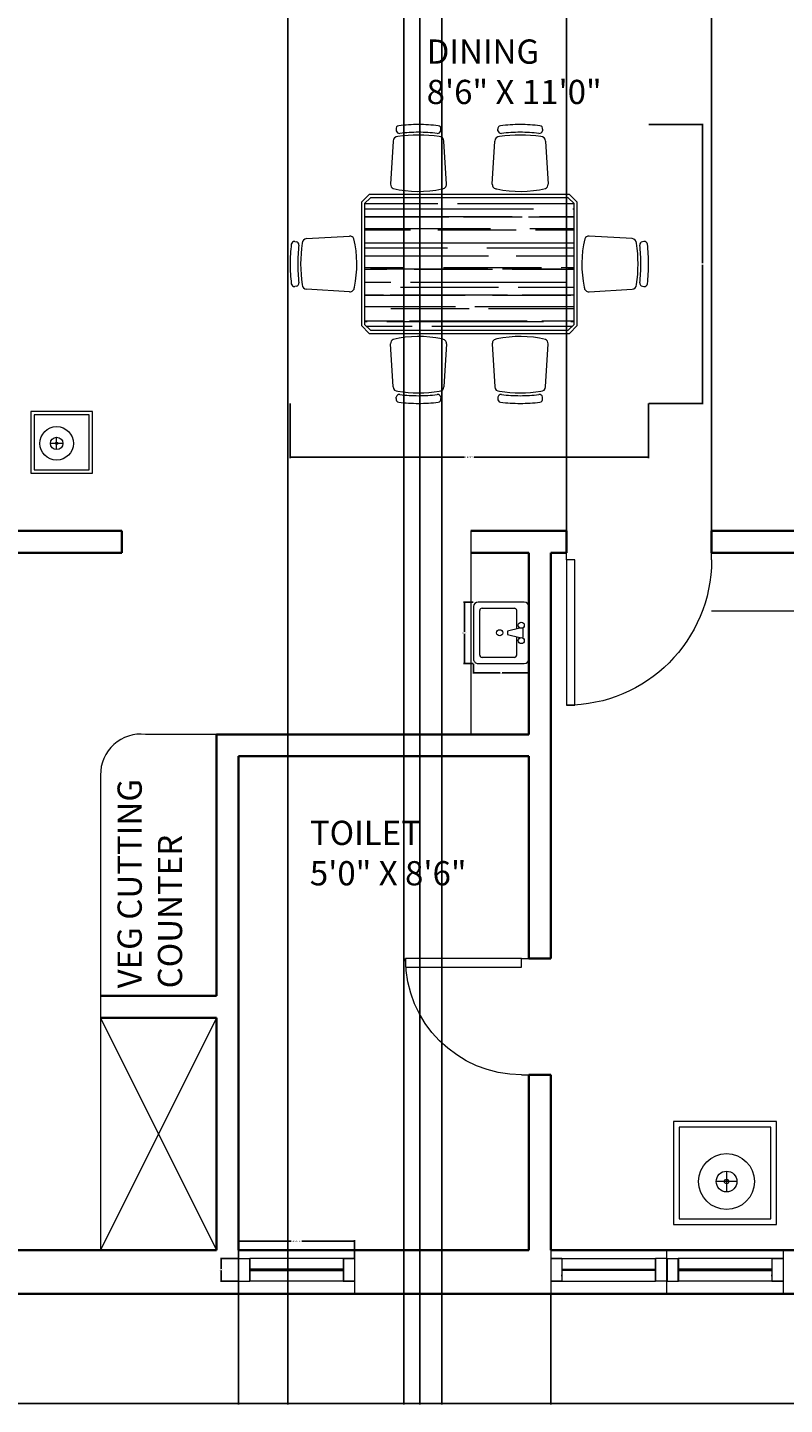
# Model space of a CAD drawing. Units: inches. Extents: x 1723 to 2209, y 1326 to 1810.
# Tile 4 of 6: x 1901 to 2057, y 1326 to 1610. Entities that reach past the tile are written whole.
import ezdxf

# ---------------------------------------------------------------- set-up
doc = ezdxf.new("R2010")
doc.units = ezdxf.units.IN
doc.layers.get('Defpoints').update_dxf_attribs({"color": 255})
for name, color, linetype, lineweight in [('A-ANNO-DIMS', 2, 'Continuous', 18), ('A-ANNO-TEXT', 7, 'Continuous', 18), ('A-AREA-IDEN', 7, 'Continuous', 18), ('A-DOOR', 3, 'Continuous', 18), ('A-FLOR-CASE', 9, 'Continuous', 18), ('A-FLOR-FIXT', 9, 'Continuous', 18), ('A-FURN', 8, 'Continuous', 13), ('A-GLAZ', 4, 'Continuous', 18), ('A-WALL', 7, 'Continuous', 35), ('muebles', 255, 'Continuous', 0), ('Sliding Door', 3, 'Continuous', 18)]:
    doc.layers.add(name, color=color, linetype=linetype, lineweight=lineweight)
doc.styles.get("Standard").update_dxf_attribs({"font": 'arial.ttf'})
doc.dimstyles.get("Standard").update_dxf_attribs({"dimtxt": 0.18, "dimasz": 0.18, "dimexe": 0.18, "dimexo": 0.0625, "dimgap": 0.09, "dimtad": 0, "dimtih": 1, "dimtoh": 1, "dimdec": 4, "dimzin": 0, "dimdsep": 46, "dimtxsty": 'Standard', "dimcen": 0.09, "dimadec": 0, "dimazin": 0, "dimtfac": 1, "dimtdec": 4, "dimtofl": 0, "dimtmove": 0, "dimatfit": 3, "dimfxl": 1, "dimtolj": 1, "dimtzin": 0, "dimarcsym": 0})

# ---------------------------------------------------------------- blocks, each defined once
blk = doc.blocks.new('50')
at = {"layer": 'muebles'}
for p, q in [((377.0913, 232.4684), (377.0744, 232.1891)), ((377.1098, 232.5445), (377.1113, 232.5346)), ((377.3997, 232.5346), (377.4011, 232.5445)), ((377.4366, 232.1891), (377.4197, 232.4684)), ((377.7344, 232.1891), (377.7513, 232.4684)), ((377.7713, 232.5346), (377.7698, 232.5445)), ((378.0611, 232.5445), (378.0597, 232.5346)), ((378.0797, 232.4684), (378.0966, 232.1891)), ((376.9355, 232.1209), (376.8855, 232.0709)), ((378.2355, 232.1209), (376.9355, 232.1209)), ((378.2855, 232.0709), (378.2355, 232.1209)), ((376.8855, 232.0709), (376.8855, 231.2709)), ((376.9438, 232.1009), (376.9055, 232.0627)), ((376.9055, 232.0627), (376.9055, 231.2792)), ((376.9055, 232.029), (378.0028, 232.029)), ((376.9061, 232.0633), (377.3805, 232.0633)), ((378.2272, 232.1009), (376.9438, 232.1009)), ((377.5075, 232.0633), (378.2648, 232.0633)), ((378.2655, 232.0627), (378.2272, 232.1009)), ((378.2568, 232.029), (378.2655, 232.029)), ((378.2655, 231.2792), (378.2655, 232.0627)), ((378.2855, 231.2709), (378.2855, 232.0709)), ((376.9055, 231.9782), (377.8631, 231.9782)), ((376.9055, 231.9769), (377.4516, 231.9769)), ((377.5469, 231.9769), (377.9279, 231.9769)), ((377.9698, 231.9769), (378.2655, 231.9769)), ((378.0409, 231.9782), (378.2655, 231.9782)), ((376.5287, 231.8351), (376.8081, 231.8521)), ((376.9055, 231.902), (377.7234, 231.902)), ((376.9055, 231.8931), (377.2027, 231.8931)), ((377.3805, 231.8931), (377.8885, 231.8931)), ((377.9774, 231.902), (378.2655, 231.902)), ((378.0155, 231.8931), (378.2655, 231.8931)), ((378.6423, 231.8351), (378.3629, 231.8521)), ((376.4526, 231.8166), (376.4625, 231.8151)), ((376.9055, 231.808), (377.5786, 231.808)), ((376.9055, 231.808), (377.2281, 231.808)), ((376.9055, 231.775), (377.444, 231.775)), ((377.3551, 231.808), (378.2655, 231.808)), ((377.6739, 231.808), (378.0549, 231.808)), ((377.698, 231.775), (378.2655, 231.775)), ((378.0968, 231.808), (378.2655, 231.808)), ((378.7183, 231.8166), (378.7084, 231.8151)), ((376.9055, 231.7229), (377.7107, 231.7229)), ((377.8885, 231.7229), (378.2655, 231.7229)), ((376.9055, 231.648), (377.1646, 231.648)), ((376.9055, 231.6378), (377.0503, 231.6378)), ((376.9436, 231.6391), (377.7056, 231.6391)), ((377.2281, 231.6378), (377.7361, 231.6378)), ((377.4186, 231.648), (378.0536, 231.648)), ((377.8009, 231.6391), (378.1819, 231.6391)), ((377.8631, 231.6378), (378.2655, 231.6378)), ((378.1806, 231.648), (378.2655, 231.648)), ((378.2238, 231.6391), (378.2655, 231.6391)), ((376.4625, 231.5267), (376.4526, 231.5253)), ((376.8081, 231.4898), (376.5287, 231.5067)), ((376.9055, 231.5528), (377.0757, 231.5528)), ((377.1392, 231.521), (377.7742, 231.521)), ((377.2027, 231.5528), (378.2187, 231.5528)), ((377.9012, 231.521), (378.2655, 231.521)), ((378.3629, 231.4898), (378.6423, 231.5067)), ((378.7084, 231.5267), (378.7183, 231.5253)), ((376.9055, 231.4702), (377.0287, 231.4702)), ((376.9055, 231.4677), (377.5583, 231.4677)), ((376.9055, 231.394), (377.4948, 231.394)), ((377.0706, 231.4702), (377.8326, 231.4702)), ((377.6218, 231.394), (378.2655, 231.394)), ((377.7361, 231.4677), (378.2441, 231.4677)), ((377.9279, 231.4702), (378.2655, 231.4702)), ((377.0757, 231.3826), (377.5837, 231.3826)), ((377.7107, 231.3826), (378.2655, 231.3826)), ((376.8855, 231.2709), (376.9355, 231.2209)), ((376.9055, 231.3013), (377.1557, 231.3013)), ((376.9055, 231.2975), (376.9233, 231.2975)), ((376.9055, 231.2792), (376.9438, 231.2409)), ((376.9177, 231.267), (377.2154, 231.267)), ((376.9355, 231.2209), (378.2355, 231.2209)), ((376.9438, 231.2409), (378.2272, 231.2409)), ((377.0503, 231.2975), (378.0663, 231.2975)), ((377.1976, 231.3013), (377.9596, 231.3013)), ((377.3424, 231.267), (378.2533, 231.267)), ((378.0549, 231.3013), (378.2655, 231.3013)), ((378.2272, 231.2409), (378.2655, 231.2792)), ((378.2355, 231.2209), (378.2855, 231.2709)), ((378.2441, 231.2975), (378.2655, 231.2975)), ((377.0913, 230.8734), (377.0744, 231.1528)), ((377.4366, 231.1528), (377.4197, 230.8734)), ((377.7344, 231.1528), (377.7513, 230.8734)), ((378.0797, 230.8734), (378.0966, 231.1528)), ((377.1098, 230.7974), (377.1113, 230.8073)), ((377.3997, 230.8073), (377.4011, 230.7974)), ((377.7713, 230.8073), (377.7698, 230.7974)), ((378.0611, 230.7974), (378.0597, 230.8073))]:
    blk.add_line(p, q, dxfattribs=at)
for centre, radius, start, end in [((377.1296, 232.5474), 0.02, 97.08312, 188.20608), ((377.2555, 231.5346), 1.0405, 90, 97.08312), ((377.2555, 231.5346), 1.0405, 82.91688, 90), ((377.3813, 232.5474), 0.02, 351.79392, 82.91688), ((377.7896, 232.5474), 0.02, 97.08312, 188.20608), ((377.9155, 231.5346), 1.0405, 90, 97.08312), ((377.9155, 231.5346), 1.0405, 82.91688, 90), ((378.0413, 232.5474), 0.02, 351.79392, 82.91688), ((377.1212, 232.4669), 0.03, 90, 177.06433), ((377.1311, 232.5375), 0.02, 188.20608, 277.072), ((377.2555, 231.566), 0.9405, 81.79392, 98.20608), ((377.2555, 231.5346), 0.9905, 90, 97.072), ((377.2555, 231.5346), 0.9905, 82.928, 90), ((377.3799, 232.5375), 0.02, 262.928, 351.79392), ((377.3897, 232.4669), 0.03, 2.93567, 90), ((377.7812, 232.4669), 0.03, 90, 177.06433), ((377.7911, 232.5375), 0.02, 188.20608, 277.072), ((377.9155, 231.566), 0.9405, 81.79392, 98.20608), ((377.9155, 231.5346), 0.9905, 90, 97.072), ((377.9155, 231.5346), 0.9905, 82.928, 90), ((378.0399, 232.5375), 0.02, 262.928, 351.79392), ((378.0497, 232.4669), 0.03, 2.93567, 90), ((377.1043, 232.1875), 0.03, 177.06433, 245.0354), ((377.2555, 232.8704), 0.7287, 257.00787, 281.97247), ((377.4066, 232.1875), 0.03, 270, 2.93567), ((377.7643, 232.1875), 0.03, 177.06433, 270), ((377.9155, 232.8704), 0.7287, 258.02753, 282.99213), ((378.0666, 232.1875), 0.03, 294.9646, 2.93567), ((376.8096, 231.8221), 0.03, 24.9646, 92.93567), ((378.3613, 231.8221), 0.03, 87.06433, 155.0354), ((377.4625, 231.6709), 1.0405, 172.91688, 180), ((376.4498, 231.7968), 0.02, 81.79392, 172.91688), ((376.4597, 231.7954), 0.02, 352.928, 81.79392), ((377.4625, 231.6709), 0.9905, 172.928, 180), ((377.4311, 231.6709), 0.9405, 171.79392, 188.20608), ((376.5302, 231.8052), 0.03, 92.93567, 180), ((376.1268, 231.6709), 0.7287, 348.02753, 12.99213), ((379.0442, 231.6709), 0.7287, 167.00787, 191.97247), ((378.6407, 231.8052), 0.03, 0, 87.06433), ((377.7398, 231.6709), 0.9405, 351.79392, 8.20608), ((378.7113, 231.7954), 0.02, 98.20608, 187.072), ((377.7084, 231.6709), 0.9905, 360, 7.072), ((378.7212, 231.7968), 0.02, 7.08312, 98.20608), ((377.7084, 231.6709), 1.0405, 360, 7.08312), ((377.4625, 231.6709), 1.0405, 180, 187.08312), ((377.4625, 231.6709), 0.9905, 180, 187.072), ((377.7084, 231.6709), 0.9905, 352.928, 0), ((377.7084, 231.6709), 1.0405, 352.91688, 0), ((376.4498, 231.5451), 0.02, 187.08312, 278.20608), ((376.4597, 231.5465), 0.02, 278.20608, 7.072), ((376.5302, 231.5367), 0.03, 180, 267.06433), ((376.8096, 231.5198), 0.03, 267.06433, 0), ((378.3613, 231.5198), 0.03, 180, 272.93567), ((378.6407, 231.5367), 0.03, 272.93567, 0), ((378.7113, 231.5465), 0.02, 172.928, 261.79392), ((378.7212, 231.5451), 0.02, 261.79392, 352.91688), ((377.1043, 231.1544), 0.03, 114.9646, 182.93567), ((377.2555, 230.4715), 0.7287, 78.02753, 102.99213), ((377.4066, 231.1544), 0.03, 357.06433, 90), ((377.7643, 231.1544), 0.03, 90, 182.93567), ((377.9155, 230.4715), 0.7287, 77.00787, 101.97247), ((378.0666, 231.1544), 0.03, 357.06433, 65.0354), ((377.1212, 230.875), 0.03, 182.93567, 270), ((377.3897, 230.875), 0.03, 270, 357.06433), ((377.7812, 230.875), 0.03, 182.93567, 270), ((378.0497, 230.875), 0.03, 270, 357.06433), ((377.1296, 230.7945), 0.02, 171.79392, 262.91688), ((377.1311, 230.8044), 0.02, 82.928, 171.79392), ((377.2555, 231.7759), 0.9405, 261.79392, 278.20608), ((377.2555, 231.8072), 1.0405, 262.91688, 270), ((377.2555, 231.8072), 0.9905, 262.928, 270), ((377.2555, 231.8072), 0.9905, 270, 277.072), ((377.2555, 231.8072), 1.0405, 270, 277.08312), ((377.3799, 230.8044), 0.02, 8.20608, 97.072), ((377.3813, 230.7945), 0.02, 277.08312, 8.20608), ((377.7896, 230.7945), 0.02, 171.79392, 262.91688), ((377.7911, 230.8044), 0.02, 82.928, 171.79392), ((377.9155, 231.7759), 0.9405, 261.79392, 278.20608), ((377.9155, 231.8072), 1.0405, 262.91688, 270), ((377.9155, 231.8072), 0.9905, 262.928, 270), ((377.9155, 231.8072), 0.9905, 270, 277.072), ((377.9155, 231.8072), 1.0405, 270, 277.08312), ((378.0399, 230.8044), 0.02, 8.20608, 97.072), ((378.0413, 230.7945), 0.02, 277.08312, 8.20608)]:
    blk.add_arc(centre, radius, start, end, dxfattribs=at)
blk = doc.blocks.new('*U39')
for p, q in [((0, 0), (0, -6)), ((24, 0), (24, -6))]:
    blk.add_line(p, q)
blk.add_lwpolyline([(0, 0), (0, 24), (1.75, 24), (1.75, 0)], close=True)
blk.add_arc((0, 0), 24, 0, 90)
blk = doc.blocks.new('*U40')
for p, q in [((0, 0), (0, -6)), ((30, 0), (30, -6))]:
    blk.add_line(p, q)
blk.add_lwpolyline([(0, 0), (0, 30), (1.75, 30), (1.75, 0)], close=True)
blk.add_arc((0, 0), 30, 0, 90)
blk = doc.blocks.new('SW')
blk.add_line((2331.37, 1559.31), (2331.37, 1550.31))
at = {"layer": 'Sliding Door'}
for p, q in [((2285.07, 1559.31), (2285.07, 1550.31)), ((2285.07, 1559.31), (2285.07, 1550.31)), ((2285.07, 1559.31), (2289.58, 1559.31)), ((2289.51, 1550.31), (2289.51, 1559.31)), ((2331.37, 1559.31), (2289.51, 1559.31)), ((2289.58, 1559.31), (2289.58, 1550.31)), ((2326.86, 1555.09), (2289.58, 1555.09)), ((2289.58, 1554.81), (2326.86, 1554.81)), ((2326.86, 1559.31), (2326.86, 1550.31)), ((2326.86, 1559.31), (2331.37, 1559.31)), ((2326.93, 1559.31), (2326.93, 1550.31)), ((2285.07, 1550.31), (2289.51, 1550.31)), ((2285.07, 1550.31), (2289.58, 1550.31)), ((2331.37, 1550.31), (2289.51, 1550.31)), ((2289.58, 1554.53), (2326.86, 1554.53)), ((2289.58, 1552.81), (2289.58, 1552.25)), ((2326.86, 1550.31), (2331.37, 1550.31)), ((2326.93, 1552.25), (2326.93, 1552.81)), ((2326.93, 1550.31), (2331.37, 1550.31))]:
    blk.add_line(p, q, dxfattribs=at)
blk = doc.blocks.new('A$C329C6BD7')
at = {"linetype": 'ByBlock'}
for p, q in [((0.47, 0.457), (0.038, 0.457)), ((0, 0.419), (0, 0.038)), ((0.07, 0.356), (0.222, 0.356)), ((0.216, 0.406), (0.292, 0.406)), ((0.216, 0.381), (0.241, 0.279)), ((0.267, 0.279), (0.292, 0.381)), ((0.286, 0.356), (0.438, 0.356)), ((0.508, 0.038), (0.508, 0.419)), ((0.051, 0.07), (0.051, 0.337)), ((0.241, 0.279), (0.267, 0.279)), ((0.457, 0.337), (0.457, 0.07)), ((0.438, 0.051), (0.07, 0.051)), ((0.038, 0), (0.47, 0))]:
    blk.add_line(p, q, dxfattribs=at)
for centre in [(0.191, 0.394), (0.318, 0.394), (0.254, 0.216)]:
    blk.add_circle(centre, 0.0254, dxfattribs=at)
for centre, radius, start, end in [((0.038, 0.419), 0.0381, 90, 180), ((0.47, 0.419), 0.0381, 0, 90), ((0.07, 0.337), 0.0191, 90, 180), ((0.438, 0.337), 0.0191, 0, 90), ((0.038, 0.038), 0.0381, 180, 270), ((0.07, 0.07), 0.0191, 180, 270), ((0.438, 0.07), 0.0191, 270, 0), ((0.47, 0.038), 0.0381, 270, 0)]:
    blk.add_arc(centre, radius, start, end, dxfattribs=at)
blk = doc.blocks.new('TABLE-END-SMALL')
for p, q in [((6.6, 6.17), (4.03, 6.17)), ((5.32, 4.88), (5.32, 7.45))]:
    blk.add_line(p, q)
for points in [[(0, 0), (12.75, 0), (12.75, 12.75), (0, 12.75)], [(0.71, 0.71), (12.04, 0.71), (12.04, 12.04), (0.71, 12.04)]]:
    blk.add_lwpolyline(points, close=True)
for radius in [3.46, 1.28, 0.266]:
    blk.add_circle((5.32, 6.17), radius)
blk = doc.blocks.new('TABLE-END-LARGE')
for p, q in [((12.41, 13.14), (12.41, 8.85)), ((10.27, 10.99), (14.56, 10.99))]:
    blk.add_line(p, q)
for points in [[(21.29, 21.29), (0, 21.29), (0, 0), (21.29, 0)], [(20.1, 20.1), (1.18, 20.1), (1.18, 1.18), (20.1, 1.18)]]:
    blk.add_lwpolyline(points, close=True)
for radius in [5.77, 2.14, 0.445]:
    blk.add_circle((12.41, 10.99), radius)
blk = doc.blocks.new('*D55')
at = {"layer": 'A-ANNO-DIMS', "color": 0, "lineweight": -2, "transparency": 16777216}
for p, q in [((1944.14, 1356.04), (1944.14, 1359.75)), ((1944.32, 1359.57), (1955, 1359.57)), ((1967.91, 1359.57), (1957.23, 1359.57)), ((1968.09, 1356.04), (1968.09, 1359.75))]:
    blk.add_line(p, q, dxfattribs=at)
at = {"layer": 'A-ANNO-DIMS', "color": 0, "transparency": 16777216}
for points in [[(1944.32, 1359.6), (1944.32, 1359.54), (1944.14, 1359.57)], [(1967.91, 1359.6), (1967.91, 1359.54), (1968.09, 1359.57)]]:
    blk.add_solid(points, dxfattribs=at)
at = {"layer": 'Defpoints', "color": 0, "transparency": 16777216}
for p in [(1968.09, 1359.57), (1944.14, 1355.98), (1968.09, 1355.98)]:
    blk.add_point(p, dxfattribs=at)
at = {"layer": 'A-ANNO-DIMS', "color": 0, "transparency": 16777216, "insert": (1956.12, 1359.57), "char_height": 0.18, "attachment_point": 5}
blk.add_mtext('\\A1;WINDOW 24 TYP.', dxfattribs=at)
blk = doc.blocks.new('*D56')
at = {"layer": 'A-ANNO-DIMS', "color": 0, "lineweight": -2, "transparency": 16777216}
for p, q in [((1944.08, 1355.98), (1940.37, 1355.98)), ((1940.55, 1355.8), (1940.55, 1353.83)), ((1940.55, 1351.5), (1940.55, 1353.47)), ((1944.08, 1351.32), (1940.37, 1351.32))]:
    blk.add_line(p, q, dxfattribs=at)
at = {"layer": 'A-ANNO-DIMS', "color": 0, "transparency": 16777216}
for points in [[(1940.52, 1355.8), (1940.58, 1355.8), (1940.55, 1355.98)], [(1940.52, 1351.5), (1940.58, 1351.5), (1940.55, 1351.32)]]:
    blk.add_solid(points, dxfattribs=at)
at = {"layer": 'Defpoints', "color": 0, "transparency": 16777216}
for p in [(1940.55, 1355.98), (1944.14, 1355.98), (1944.14, 1351.32)]:
    blk.add_point(p, dxfattribs=at)
at = {"layer": 'A-ANNO-DIMS', "color": 0, "transparency": 16777216, "insert": (1940.55, 1353.65), "char_height": 0.18, "attachment_point": 5}
blk.add_mtext('\\A1;5 TYP.', dxfattribs=at)
blk = doc.blocks.new('*D85')
at = {"layer": 'A-ANNO-DIMS', "color": 0, "lineweight": -2, "transparency": 16777216}
for p, q in [((1954.77, 1532.46), (1954.77, 1521.23)), ((2028.84, 1532.46), (2028.84, 1521.23)), ((1954.95, 1521.41), (1990.83, 1521.41)), ((2028.66, 1521.41), (1992.77, 1521.41))]:
    blk.add_line(p, q, dxfattribs=at)
at = {"layer": 'A-ANNO-DIMS', "color": 0, "transparency": 16777216}
for points in [[(1954.95, 1521.44), (1954.95, 1521.38), (1954.77, 1521.41)], [(2028.66, 1521.44), (2028.66, 1521.38), (2028.84, 1521.41)]]:
    blk.add_solid(points, dxfattribs=at)
at = {"layer": 'Defpoints', "color": 0, "transparency": 16777216}
for p in [(1954.77, 1532.52), (2028.84, 1532.52), (2028.84, 1521.41)]:
    blk.add_point(p, dxfattribs=at)
at = {"layer": 'A-ANNO-DIMS', "color": 0, "transparency": 16777216, "insert": (1991.8, 1521.41), "char_height": 0.18, "attachment_point": 5}
blk.add_mtext('\\A1;DINING SET 74', dxfattribs=at)
blk = doc.blocks.new('*D86')
at = {"layer": 'A-ANNO-DIMS', "color": 0, "lineweight": -2, "transparency": 16777216}
for p, q in [((2028.9, 1590.08), (2040.13, 1590.08)), ((2039.95, 1589.9), (2039.95, 1561.48)), ((2039.95, 1532.7), (2039.95, 1561.12)), ((2028.9, 1532.52), (2040.13, 1532.52))]:
    blk.add_line(p, q, dxfattribs=at)
at = {"layer": 'A-ANNO-DIMS', "color": 0, "transparency": 16777216}
for points in [[(2039.92, 1589.9), (2039.98, 1589.9), (2039.95, 1590.08)], [(2039.92, 1532.7), (2039.98, 1532.7), (2039.95, 1532.52)]]:
    blk.add_solid(points, dxfattribs=at)
at = {"layer": 'Defpoints', "color": 0, "transparency": 16777216}
for p in [(2028.84, 1590.08), (2039.95, 1590.08), (2028.84, 1532.52)]:
    blk.add_point(p, dxfattribs=at)
at = {"layer": 'A-ANNO-DIMS', "color": 0, "transparency": 16777216, "insert": (2039.95, 1561.3), "char_height": 0.18, "attachment_point": 5}
blk.add_mtext('\\A1;58', dxfattribs=at)
blk = doc.blocks.new('*D91')
at = {"layer": 'A-ANNO-DIMS', "color": 0, "lineweight": -2, "transparency": 16777216}
for p, q in [((1992.61, 1491.5), (1990.59, 1491.5)), ((1990.77, 1491.32), (1990.77, 1485.34)), ((1990.77, 1478.98), (1990.77, 1484.97)), ((1992.61, 1478.8), (1990.59, 1478.8))]:
    blk.add_line(p, q, dxfattribs=at)
at = {"layer": 'A-ANNO-DIMS', "color": 0, "transparency": 16777216}
for points in [[(1990.74, 1491.32), (1990.8, 1491.32), (1990.77, 1491.5)], [(1990.74, 1478.98), (1990.8, 1478.98), (1990.77, 1478.8)]]:
    blk.add_solid(points, dxfattribs=at)
at = {"layer": 'Defpoints', "color": 0, "transparency": 16777216}
for p in [(1992.67, 1491.5), (1990.77, 1478.8), (1992.67, 1478.8)]:
    blk.add_point(p, dxfattribs=at)
at = {"layer": 'A-ANNO-DIMS', "color": 0, "transparency": 16777216, "insert": (1990.77, 1485.15), "char_height": 0.18, "attachment_point": 5}
blk.add_mtext('\\A1;BASIN 13', dxfattribs=at)
blk = doc.blocks.new('*D92')
at = {"layer": 'A-ANNO-DIMS', "color": 0, "lineweight": -2, "transparency": 16777216}
for p, q in [((1992.67, 1478.74), (1992.67, 1476.72)), ((2004.1, 1478.74), (2004.1, 1476.72)), ((1992.85, 1476.9), (1998.2, 1476.9)), ((2003.92, 1476.9), (1998.58, 1476.9))]:
    blk.add_line(p, q, dxfattribs=at)
at = {"layer": 'A-ANNO-DIMS', "color": 0, "transparency": 16777216}
for points in [[(1992.85, 1476.93), (1992.85, 1476.87), (1992.67, 1476.9)], [(2003.92, 1476.93), (2003.92, 1476.87), (2004.1, 1476.9)]]:
    blk.add_solid(points, dxfattribs=at)
at = {"layer": 'Defpoints', "color": 0, "transparency": 16777216}
for p in [(1992.67, 1478.8), (2004.1, 1478.8), (2004.1, 1476.9)]:
    blk.add_point(p, dxfattribs=at)
at = {"layer": 'A-ANNO-DIMS', "color": 0, "transparency": 16777216, "insert": (1998.39, 1476.9), "char_height": 0.18, "attachment_point": 5}
blk.add_mtext('\\A1;11', dxfattribs=at)
blk = doc.blocks.new('*D96')
at = {"layer": 'A-ANNO-DIMS', "color": 0, "lineweight": -2, "transparency": 16777216}
for p, q in [((1944.1, 1357.63), (1944.1, 1325.84)), ((1788.1, 1348.63), (1788.1, 1325.84)), ((1788.28, 1326.02), (1865.82, 1326.02)), ((1943.92, 1326.02), (1866.38, 1326.02))]:
    blk.add_line(p, q, dxfattribs=at)
at = {"layer": 'A-ANNO-DIMS', "color": 0, "transparency": 16777216}
for points in [[(1788.28, 1326.05), (1788.28, 1325.99), (1788.1, 1326.02)], [(1943.92, 1326.05), (1943.92, 1325.99), (1944.1, 1326.02)]]:
    blk.add_solid(points, dxfattribs=at)
at = {"layer": 'Defpoints', "color": 0, "transparency": 16777216}
for p in [(1944.1, 1357.69), (1788.1, 1348.69), (1944.1, 1326.02)]:
    blk.add_point(p, dxfattribs=at)
at = {"layer": 'A-ANNO-DIMS', "color": 0, "transparency": 16777216, "insert": (1866.1, 1326.02), "char_height": 0.18, "attachment_point": 5}
blk.add_mtext('\\A1;156', dxfattribs=at)
blk = doc.blocks.new('*D97')
at = {"layer": 'A-ANNO-DIMS', "color": 0, "lineweight": -2, "transparency": 16777216}
for p, q in [((1944.1, 1357.63), (1944.1, 1325.84)), ((2008.6, 1348.63), (2008.6, 1325.84)), ((1944.28, 1326.02), (1976.03, 1326.02)), ((2008.42, 1326.02), (1976.68, 1326.02))]:
    blk.add_line(p, q, dxfattribs=at)
at = {"layer": 'A-ANNO-DIMS', "color": 0, "transparency": 16777216}
for points in [[(1944.28, 1326.05), (1944.28, 1325.99), (1944.1, 1326.02)], [(2008.42, 1326.05), (2008.42, 1325.99), (2008.6, 1326.02)]]:
    blk.add_solid(points, dxfattribs=at)
at = {"layer": 'Defpoints', "color": 0, "transparency": 16777216}
for p in [(1944.1, 1357.69), (2008.6, 1348.69), (2008.6, 1326.02)]:
    blk.add_point(p, dxfattribs=at)
at = {"layer": 'A-ANNO-DIMS', "color": 0, "transparency": 16777216, "insert": (1976.35, 1326.02), "char_height": 0.18, "attachment_point": 5}
blk.add_mtext('\\A1;64.5', dxfattribs=at)
blk = doc.blocks.new('*D98')
at = {"layer": 'A-ANNO-DIMS', "color": 0, "lineweight": -2, "transparency": 16777216}
for p, q in [((2152.6, 1357.63), (2152.6, 1325.84)), ((2008.6, 1348.63), (2008.6, 1325.84)), ((2008.78, 1326.02), (2080.32, 1326.02)), ((2152.42, 1326.02), (2080.88, 1326.02))]:
    blk.add_line(p, q, dxfattribs=at)
at = {"layer": 'A-ANNO-DIMS', "color": 0, "transparency": 16777216}
for points in [[(2008.78, 1326.05), (2008.78, 1325.99), (2008.6, 1326.02)], [(2152.42, 1326.05), (2152.42, 1325.99), (2152.6, 1326.02)]]:
    blk.add_solid(points, dxfattribs=at)
at = {"layer": 'Defpoints', "color": 0, "transparency": 16777216}
for p in [(2152.6, 1357.69), (2008.6, 1348.69), (2152.6, 1326.02)]:
    blk.add_point(p, dxfattribs=at)
at = {"layer": 'A-ANNO-DIMS', "color": 0, "transparency": 16777216, "insert": (2080.6, 1326.02), "char_height": 0.18, "attachment_point": 5}
blk.add_mtext('\\A1;144', dxfattribs=at)
blk = doc.blocks.new('*D107')
at = {"layer": 'A-ANNO-DIMS', "color": 0, "lineweight": -2, "transparency": 16777216}
for p, q in [((2011.84, 1506.25), (2011.84, 1809.54)), ((2012.02, 1809.36), (2026.63, 1809.36)), ((2041.66, 1809.36), (2027.06, 1809.36)), ((2041.84, 1506.25), (2041.84, 1809.54))]:
    blk.add_line(p, q, dxfattribs=at)
at = {"layer": 'A-ANNO-DIMS', "color": 0, "transparency": 16777216}
for points in [[(2012.02, 1809.39), (2012.02, 1809.33), (2011.84, 1809.36)], [(2041.66, 1809.39), (2041.66, 1809.33), (2041.84, 1809.36)]]:
    blk.add_solid(points, dxfattribs=at)
at = {"layer": 'Defpoints', "color": 0, "transparency": 16777216}
for p in [(2041.84, 1809.36), (2011.84, 1506.19), (2041.84, 1506.19)]:
    blk.add_point(p, dxfattribs=at)
at = {"layer": 'A-ANNO-DIMS', "color": 0, "transparency": 16777216, "insert": (2026.84, 1809.36), "char_height": 0.18, "attachment_point": 5}
blk.add_mtext('\\A1;30', dxfattribs=at)
blk = doc.blocks.new('*D108')
at = {"layer": 'A-ANNO-DIMS', "color": 0, "lineweight": -2, "transparency": 16777216}
for p, q in [((1954.3, 1671.13), (1954.3, 1325.84)), ((1978.3, 1671.13), (1978.3, 1325.84)), ((1954.48, 1326.02), (1966.08, 1326.02)), ((1978.12, 1326.02), (1966.52, 1326.02))]:
    blk.add_line(p, q, dxfattribs=at)
at = {"layer": 'A-ANNO-DIMS', "color": 0, "transparency": 16777216}
for points in [[(1954.48, 1326.05), (1954.48, 1325.99), (1954.3, 1326.02)], [(1978.12, 1326.05), (1978.12, 1325.99), (1978.3, 1326.02)]]:
    blk.add_solid(points, dxfattribs=at)
at = {"layer": 'Defpoints', "color": 0, "transparency": 16777216}
for p in [(1954.3, 1671.19), (1978.3, 1671.19), (1978.3, 1326.02)]:
    blk.add_point(p, dxfattribs=at)
at = {"layer": 'A-ANNO-DIMS', "color": 0, "transparency": 16777216, "insert": (1966.3, 1326.02), "char_height": 0.18, "attachment_point": 5}
blk.add_mtext('\\A1;24', dxfattribs=at)
blk = doc.blocks.new('*D109')
at = {"layer": 'A-ANNO-DIMS', "color": 0, "lineweight": -2, "transparency": 16777216}
for p, q in [((1981.6, 1777.63), (1981.6, 1325.84)), ((1986.1, 1777.63), (1986.1, 1325.84)), ((1981.78, 1326.02), (1983.6, 1326.02)), ((1985.92, 1326.02), (1984.11, 1326.02))]:
    blk.add_line(p, q, dxfattribs=at)
at = {"layer": 'A-ANNO-DIMS', "color": 0, "transparency": 16777216}
for points in [[(1981.78, 1326.05), (1981.78, 1325.99), (1981.6, 1326.02)], [(1985.92, 1326.05), (1985.92, 1325.99), (1986.1, 1326.02)]]:
    blk.add_solid(points, dxfattribs=at)
at = {"layer": 'Defpoints', "color": 0, "transparency": 16777216}
for p in [(1981.6, 1777.69), (1986.1, 1777.69), (1986.1, 1326.02)]:
    blk.add_point(p, dxfattribs=at)
at = {"layer": 'A-ANNO-DIMS', "color": 0, "transparency": 16777216, "insert": (1983.85, 1326.02), "char_height": 0.18, "attachment_point": 5}
blk.add_mtext('\\A1;4.5', dxfattribs=at)

msp = doc.modelspace()

# ---------------------------------------------------------------- linework, layer by layer
at = {"layer": 'A-FLOR-CASE'}
for p, q in [((1992.1032, 1506.1915), (1992.1032, 1464.1915)), ((2041.8437, 1501.6915), (2151.6826, 1501.6915)), ((2041.8437, 1489.6915), (2113.9849, 1489.6915)), ((1939.6032, 1405.6915), (1915.6032, 1357.6915)), ((1915.6032, 1405.6915), (1939.6032, 1357.6915)), ((1915.6032, 1405.6915), (1915.6032, 1357.6915))]:
    msp.add_line(p, q, dxfattribs=at)
for points in [[(1939.6032, 1464.1915), (1924.9109, 1464.1915)], [(1915.6032, 1455.8923), (1915.6032, 1405.6915)]]:
    msp.add_lwpolyline(points, dxfattribs=at)
msp.add_arc((1924.001, 1455.8429), 8.398, 83.780478, 180.337239, dxfattribs=at)
at = {"layer": 'A-GLAZ'}
for points in [[(1944.0935, 1357.6915), (1968.0935, 1357.6915), (1968.0935, 1348.6915), (1944.0935, 1348.6915)], [(2032.6043, 1357.6915), (2008.6043, 1357.6915), (2008.6043, 1348.6915), (2032.6043, 1348.6915)], [(2032.6043, 1357.6915), (2056.6043, 1357.6915), (2056.6043, 1348.6915), (2032.6043, 1348.6915)]]:
    msp.add_lwpolyline(points, close=True, dxfattribs=at)
at = {"layer": 'A-WALL'}
for p, q in [((1920.017, 1506.1915), (1816.6032, 1506.1915)), ((1920.017, 1501.6915), (1920.017, 1506.1915)), ((2011.8437, 1506.1915), (1992.1032, 1506.1915)), ((2011.8437, 1501.6915), (2011.8437, 1506.1915)), ((2176.6032, 1506.1915), (2041.8437, 1506.1915)), ((2041.8437, 1501.6915), (2041.8437, 1506.1915)), ((1920.017, 1501.6915), (1797.1032, 1501.6915)), ((2004.1032, 1501.6915), (1992.1032, 1501.6915)), ((2004.1032, 1501.6915), (2004.1032, 1464.1915)), ((2008.6032, 1501.6915), (2008.6032, 1417.8977)), ((2011.8437, 1501.6915), (2008.6032, 1501.6915)), ((2176.6032, 1501.6915), (2041.8437, 1501.6915)), ((2004.1032, 1464.1915), (1939.6032, 1464.1915)), ((1939.6032, 1464.1915), (1939.6032, 1410.1915)), ((2004.1032, 1459.6915), (1944.1032, 1459.6915)), ((1944.1032, 1459.6915), (1944.1032, 1357.6915)), ((2004.1032, 1459.6915), (2004.1032, 1417.8977)), ((2004.1032, 1417.8977), (2008.6032, 1417.8977)), ((1939.6032, 1410.1915), (1915.6032, 1410.1915)), ((1939.6032, 1405.6915), (1915.6032, 1405.6915)), ((1939.6032, 1405.6915), (1939.6032, 1357.6915)), ((2004.1032, 1393.8977), (2008.6032, 1393.8977)), ((2004.1032, 1393.8977), (2004.1032, 1357.6915)), ((2008.6032, 1393.8977), (2008.6032, 1357.6915)), ((1939.6032, 1357.6915), (1797.1032, 1357.6915)), ((2004.1032, 1357.6915), (1944.1032, 1357.6915)), ((2176.6032, 1357.6915), (2008.6032, 1357.6915))]:
    msp.add_line(p, q, dxfattribs=at)
msp.add_lwpolyline([(2185.6032, 1576.485), (2185.6032, 1348.6915), (1788.1032, 1348.6915), (1788.1032, 1506.1915)], dxfattribs=at)

# ---------------------------------------------------------------- block references
at = {"layer": 'A-DOOR', "xscale": -1}
for name, p, rotation in [('*U40', (2011.8437, 1500.1915), 180), ('*U39', (2002.6032, 1417.8977), 89.99999999999936)]:
    msp.add_blockref(name, p, dxfattribs=dict(at, rotation=rotation))
at = {"layer": 'A-FLOR-FIXT', "xscale": 24.99853146885707, "yscale": 24.99853146885707, "zscale": 24.99853146885707, "rotation": 270}
msp.add_blockref('A$C329C6BD7', (1992.6738, 1491.5023), dxfattribs=at)
at = {"layer": 'A-FURN', "xscale": 31.83083264286002, "yscale": 31.83083264286002, "zscale": 31.83083264286002}
msp.add_blockref('50', (-10027.0588, -5812.978), dxfattribs=at)
at = {"layer": 'A-FURN'}
msp.add_blockref('TABLE-END-SMALL', (1901.2276, 1518.086), dxfattribs=at)
at = {"layer": 'A-FURN', "rotation": 270.0000000000014}
msp.add_blockref('TABLE-END-LARGE', (2033.9449, 1384.2788), dxfattribs=at)
at = {"layer": 'A-GLAZ', "yscale": 0.5174661543078929, "zscale": 0.5174661543078929}
for p, xscale in [((761.6905, 549.088), 0.5174661543078929), ((3215.0073, 549.088), -0.5174661543078929), ((850.2012, 549.088), 0.5174661543078929)]:
    msp.add_blockref('SW', p, dxfattribs=dict(at, xscale=xscale))

# ---------------------------------------------------------------- texts
at = {"layer": 'A-ANNO-TEXT', "insert": (1919.131, 1411.7472), "char_height": 5, "attachment_point": 1, "rotation": 90}
msp.add_mtext_dynamic_manual_height_columns('VEG CUTTING COUNTER', width=47.827282, gutter_width=12.5, heights=[0], dxfattribs=at)
at = {"layer": 'A-AREA-IDEN', "char_height": 5, "attachment_point": 1}
for s, width, insert in [('DINING\\P8\'6" X 11\'0"', 79.790232, (1982.98, 1607.6493)), ('TOILET\\P5\'0" X 8\'6"', 40.517526, (1958.8553, 1446.3482))]:
    msp.add_mtext_dynamic_manual_height_columns(s, width=width, gutter_width=12.5, heights=[0], dxfattribs=dict(at, insert=insert))

# ---------------------------------------------------------------- dimensions: what is measured, and where the dimension line sits
at = {"layer": 'A-ANNO-DIMS'}
for base, p1, p2, override, picture, middle in [((2041.8437, 1809.3615), (2011.8437, 1506.1915), (2041.8437, 1506.1915), {"dimdec": 0, "dimlfac": 1, "dimrnd": 0, "dimzin": 0, "dimdsep": 46, "dimlunit": 2}, '*D107', (2026.8437, 1809.3615)), ((1986.1032, 1326.0215), (1981.6032, 1777.6915), (1986.1032, 1777.6915), {"dimdec": 1, "dimlfac": 1, "dimrnd": 0, "dimzin": 0, "dimdsep": 46, "dimlunit": 2}, '*D109', (1983.8532, 1326.0215)), ((1978.3022, 1326.0215), (1954.3022, 1671.1915), (1978.3022, 1671.1915), {"dimdec": 0, "dimlfac": 1, "dimrnd": 0, "dimzin": 0, "dimdsep": 46, "dimlunit": 2}, '*D108', (1966.3022, 1326.0215)), ((2004.1032, 1476.8981), (1992.6738, 1478.803), (2004.1032, 1478.803), {"dimdec": 0, "dimlfac": 1, "dimrnd": 0, "dimzin": 0, "dimdsep": 46, "dimlunit": 2}, '*D92', (1998.3885, 1476.8981)), ((1944.1032, 1326.0215), (1788.1032, 1348.6915), (1944.1032, 1357.6915), {"dimdec": 0, "dimlfac": 1, "dimrnd": 0, "dimzin": 0, "dimdsep": 46, "dimlunit": 2}, '*D96', (1866.1032, 1326.0215)), ((2008.6043, 1326.0215), (1944.1032, 1357.6915), (2008.6043, 1348.6915), {"dimdec": 1, "dimlfac": 1, "dimrnd": 0, "dimzin": 0, "dimdsep": 46, "dimlunit": 2}, '*D97', (1976.3537, 1326.0215)), ((2152.6032, 1326.0215), (2008.6043, 1348.6915), (2152.6032, 1357.6915), {"dimdec": 0, "dimlfac": 1, "dimrnd": 0, "dimzin": 0, "dimdsep": 46, "dimlunit": 2}, '*D98', (2080.6037, 1326.0215))]:
    dim = msp.add_linear_dim(base=base, p1=p1, p2=p2, dimstyle='Standard', override=override, dxfattribs=at)
    dim.commit()
    dim.dimension.update_dxf_attribs({"geometry": picture, "text_midpoint": middle})
dim = msp.add_linear_dim(base=(2039.946, 1590.0824), p1=(2028.8357, 1532.5197), p2=(2028.8357, 1590.0824), angle=90, dimstyle='Standard', override={"dimdec": 0, "dimlfac": 1, "dimrnd": 0, "dimzin": 0, "dimdsep": 46, "dimlunit": 2}, dxfattribs=at)
dim.commit()
dim.dimension.update_dxf_attribs({"geometry": '*D86', "text_midpoint": (2039.946, 1561.301)})
for base, p1, p2, text, picture, middle in [((2028.8357, 1521.4094), (1954.767, 1532.5197), (2028.8357, 1532.5197), 'DINING SET <>', '*D85', (1991.8013, 1521.4094)), ((1968.0935, 1359.5713), (1944.1386, 1355.9781), (1968.0935, 1355.9781), 'WINDOW <> TYP.', '*D55', (1956.1161, 1359.5713))]:
    dim = msp.add_linear_dim(base=base, p1=p1, p2=p2, text=text, dimstyle='Standard', override={"dimdec": 0, "dimlfac": 1, "dimrnd": 0, "dimzin": 0, "dimdsep": 46, "dimlunit": 2}, dxfattribs=at)
    dim.commit()
    dim.dimension.update_dxf_attribs({"geometry": picture, "text_midpoint": middle})
for base, p1, p2, angle, text, picture, middle in [((1990.7689, 1478.803), (1992.6738, 1491.5023), (1992.6738, 1478.803), 270, 'BASIN <>', '*D91', (1990.7689, 1485.1526)), ((1940.5454, 1355.9781), (1944.1386, 1351.3209), (1944.1386, 1355.9781), 90, '<> TYP.', '*D56', (1940.5454, 1353.6495))]:
    dim = msp.add_linear_dim(base=base, p1=p1, p2=p2, angle=angle, text=text, dimstyle='Standard', override={"dimdec": 0, "dimlfac": 1, "dimrnd": 0, "dimzin": 0, "dimdsep": 46, "dimlunit": 2}, dxfattribs=at)
    dim.commit()
    dim.dimension.update_dxf_attribs({"geometry": picture, "text_midpoint": middle})

doc.saveas('drawing.dxf')
